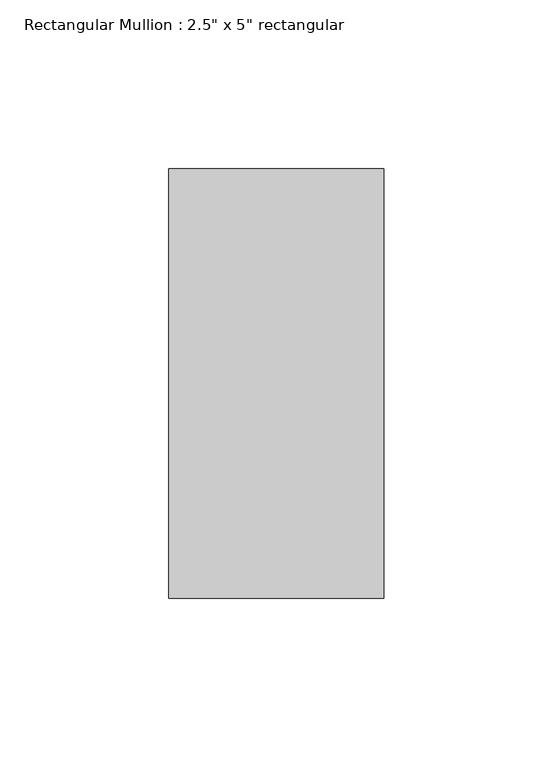
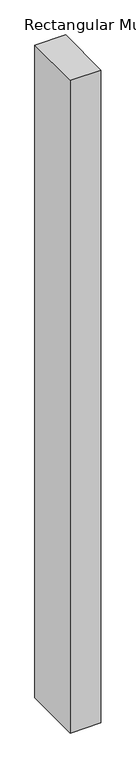
"""IFC4 building model written with IfcOpenShell, lengths in millimetres: member geometry."""

from ifc_helpers import new_model, si_unit, frame, origin, place, context, project, spatial, polyline, outline, extrude, source, transform, mapped, element, save


def member_4cf64162(model_context):
    return source(origin(), model_context, "Body", "SweptSolid", [
        extrude(outline(polyline([(0.0, 63.5), (0.0, -63.5), (-63.5, -63.5), (-63.5, 63.5), (0.0, 63.5)])), frame((0.0, 0.0, -1430.8419021), z_axis=(0.0, 0.0, 1.0), x_axis=(1.0, 0.0, 0.0)), (0.0, 0.0, 1.0), 1430.8419021),
    ])


if __name__ == "__main__":
    model = new_model("IFC4")
    model_context = context("Model", 3, world=origin())
    ifc_project = project(units=[si_unit("LENGTHUNIT", "METRE", prefix="MILLI")], contexts=[model_context])
    site = spatial("IfcSite", under=ifc_project)
    building = spatial("IfcBuilding", under=site)
    placement = place(None, origin())
    member_shape = member_4cf64162(model_context)
    element("IfcMember", 1, ObjectType="Rectangular Mullion : 2.5\" x 5\" rectangular", at=placement, inside=building, context=model_context, shape_type="MappedRepresentation", body=[
        mapped(member_shape, transform((0.0, 0.0, 0.0), x_axis=(1.0, 0.0, 0.0), y_axis=(0.0, 1.0, 0.0), z_axis=(0.0, 0.0, 1.0))),
    ])
    save(model, "model.ifc")

# Revit data of these elements
# Type "Rectangular Mullion : 2.5\" x 5\" rectangular"
#   built-in parameter 1007304 = 0.416667 (stored number, unit not read)
#   built-in parameter 1007301 = 0.104167 (stored number, unit not read)
#   built-in parameter 1007300 = 0.104167 (stored number, unit not read)
# Element 1 (IfcMember, "Rectangular Mullion : 2.5\" x 5\" rectangular")
#   Materials on its faces: "Aluminum"
# Materials
#   "Aluminum": class "Metal", colour RGB 247 247 247, transparency 0, Description = "Aluminum 6061", Cost = 0
